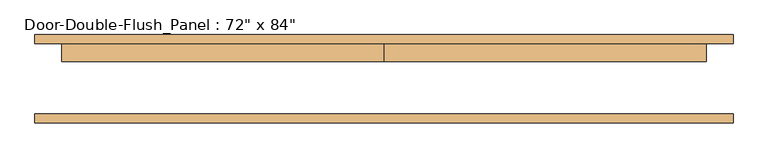
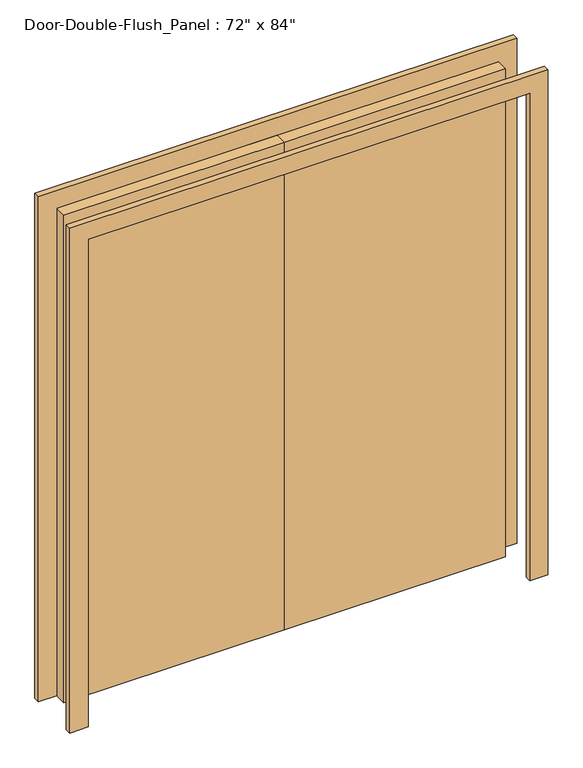
"""IFC4 building model written with IfcOpenShell, lengths in millimetres: door geometry."""

from ifc_helpers import new_model, si_unit, frame, origin, origin_with_axes, place, context, project, spatial, polyline, outline, extrude, source, transform, mapped, element, save


def door_db0c0681(model_context):
    return source(origin(), model_context, "Body", "SweptSolid", [
        extrude(outline(polyline([(2133.6, -914.4), (2133.6, 914.4), (0.0, 914.4), (0.0, 990.6), (2209.8, 990.6), (2209.8, -990.6), (0.0, -990.6), (0.0, -914.4), (2133.6, -914.4)])), frame((0.0, -125.4, 0.0), z_axis=(0.0, 1.0, 0.0), x_axis=(0.0, 0.0, 1.0)), (0.0, 0.0, 1.0), 25.4),
        extrude(outline(polyline([(2133.6, -914.4), (2133.6, 914.4), (0.0, 914.4), (0.0, 990.6), (2209.8, 990.6), (2209.8, -990.6), (0.0, -990.6), (0.0, -914.4), (2133.6, -914.4)])), frame((0.0, 100.0, 0.0), z_axis=(0.0, 1.0, 0.0), x_axis=(0.0, 0.0, 1.0)), (0.0, 0.0, 1.0), 25.4),
        extrude(outline(polyline([(0.0, 100.0), (914.4, 100.0), (914.4, 49.2), (0.0, 49.2), (0.0, 100.0)])), origin_with_axes(), (0.0, 0.0, 1.0), 2133.6),
        extrude(outline(polyline([(-914.4, 100.0), (0.0, 100.0), (0.0, 49.2), (-914.4, 49.2), (-914.4, 100.0)])), origin_with_axes(), (0.0, 0.0, 1.0), 2133.6),
    ])


if __name__ == "__main__":
    model = new_model("IFC4")
    model_context = context("Model", 3, world=origin())
    ifc_project = project(units=[si_unit("LENGTHUNIT", "METRE", prefix="MILLI")], contexts=[model_context])
    site = spatial("IfcSite", under=ifc_project)
    building = spatial("IfcBuilding", under=site)
    placement = place(None, origin())
    door_shape = door_db0c0681(model_context)
    element("IfcDoor", 1, ObjectType="Door-Double-Flush_Panel : 72\" x 84\"", at=placement, inside=building, context=model_context, shape_type="MappedRepresentation", body=[
        mapped(door_shape, transform((0.0, 0.0, 0.0), x_axis=(1.0, 0.0, 0.0), y_axis=(0.0, 1.0, 0.0), z_axis=(0.0, 0.0, 1.0))),
    ])
    save(model, "model.ifc")

# Revit data of these elements
# Type "Door-Double-Flush_Panel : 72\" x 84\""
#   Type Mark = "22"
#   Construction Type Id = "DOOR"
#   Assembly Code = "C1020"
#   Analytic Construction = "Wooden"
#   Thickness = 0' - 2"
#   Thermal Resistance (R) = 0.455703 (m²·K)/W
#   Swing Angle [instance default] = 90.00°
#   Panel Width = 3' - 0"
#   Heat Transfer Coefficient (U) = 2.19465 W/(m²·K)
#   Height = 7' - 0"
#   Trim Projection Ext = 0' - 1"
#   Trim Projection Int = 0' - 1"
#   Trim Width = 0' - 3"
#   Width = 6' - 0"
#   Define Thermal Properties by = 1
#   Panel Material = Wood - Birch - Solid Stained Light Low Gloss
#   Trim Material = Paint - Sienna
#   Visual Light Transmittance = 0
#   Solar Heat Gain Coefficient = 0
#   Function = (empty or 0)
#   Wall Closure = (empty or 0)
# Element 1 (IfcDoor, "Door-Double-Flush_Panel : 72\" x 84\"")
#   Materials on its faces: "Paint - Sienna", "Wood - Birch - Solid Stained Light Low Gloss"
# Materials
#   "Wood - Birch - Solid Stained Light Low Gloss": class "Wood", colour RGB 210 159 95, transparency 0, Cost = 0
#   "Paint - Sienna": colour RGB 118 70 51, transparency 0, Cost = 0
